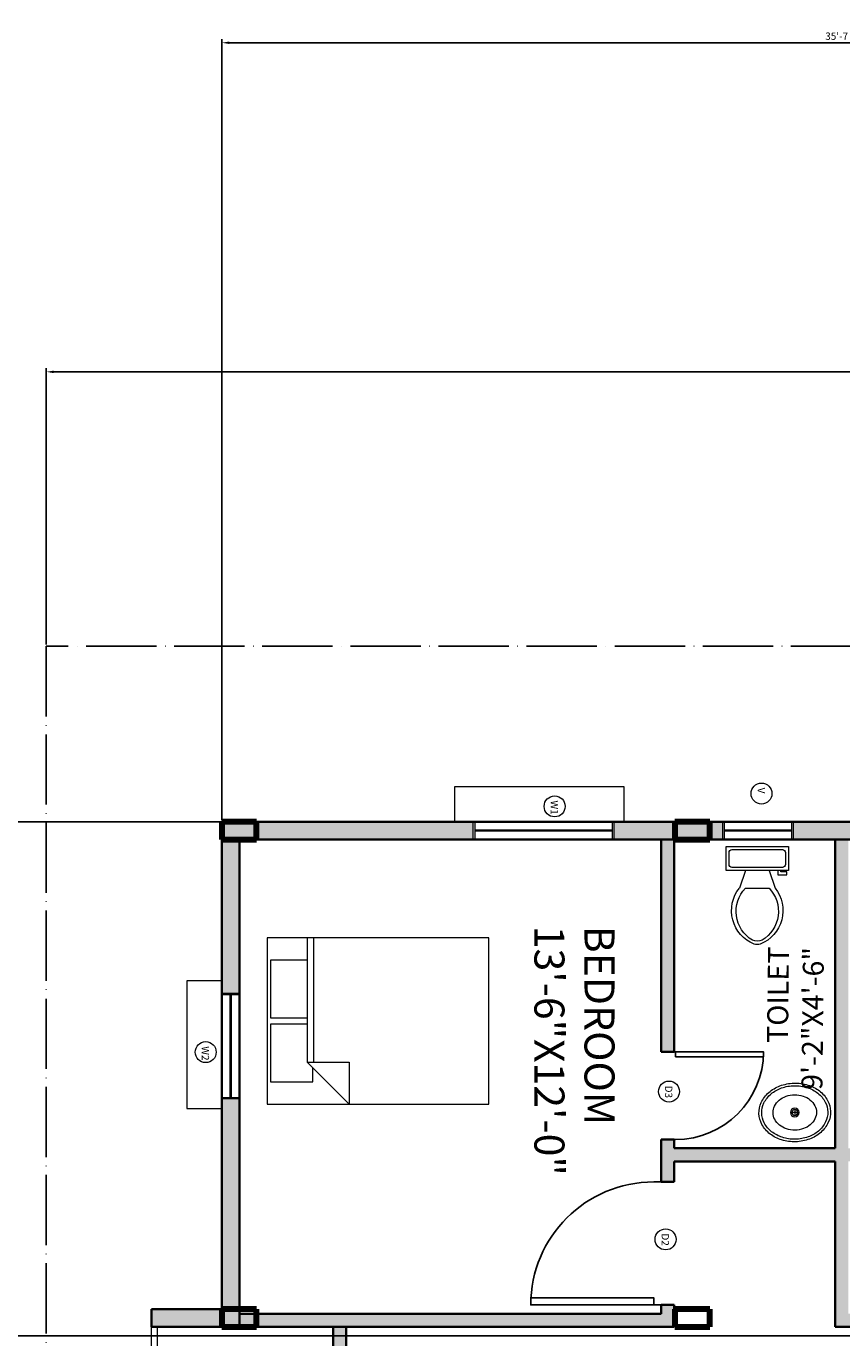
# Model space of a CAD drawing. Units: inches. Extents: x 7028582 to 7030319, y 63109697 to 63111305.
# Tile 11 of 18: x 7029168 to 7029446, y 63110857 to 63111305. Entities that reach past the tile are written whole.
import ezdxf

# ---------------------------------------------------------------- set-up
doc = ezdxf.new("R2010")
doc.units = ezdxf.units.IN
doc.linetypes.add('ACAD_ISO04W100', pattern=[30, 24, -3, 0, -3])
for name, color, linetype, lineweight in [('A-AREA-IDEN', 7, 'Continuous', 18), ('A-DOOR-IDEN', 20, 'Continuous', 13), ('A-FLOR-FIXT', 9, 'Continuous', 18), ('A-FLOR-HRAL', 5, 'Continuous', 18), ('A-GLAZ-IDEN', 20, 'Continuous', 13), ('A-WALL-PATT', 8, 'Continuous', 13), ('C-ANNO-DIMS', 7, 'Continuous', 18), ('C-PROP', 1, 'ACAD_ISO04W100', 25), ('doors', 20, 'Continuous', 25), ('furniture', 9, 'Continuous', 18), ('PILLARS', 220, 'Continuous', 100), ('S-COLS-PATT', 220, 'Continuous', 100), ('walls', 6, 'Continuous', 35), ('WINDOW SHADOW', 9, 'Continuous', 13), ('windows', 5, 'Continuous', 18)]:
    doc.layers.add(name, color=color, linetype=linetype, lineweight=lineweight)
doc.styles.get("Standard").update_dxf_attribs({"font": 'arial.ttf'})
doc.dimstyles.new('ISO-25', dxfattribs={"dimtxt": 2.5, "dimasz": 2.5, "dimexe": 1.25, "dimexo": 0.625, "dimtad": 1, "dimlunit": 4, "dimtxsty": 'Standard', "dimcen": 2.5, "dimadec": 0, "dimazin": 0, "dimtfac": 1, "dimtmove": 0, "dimatfit": 3, "dimfxl": 1, "dimarcsym": 0})

# ---------------------------------------------------------------- blocks, each defined once
blk = doc.blocks.new('*U2')
for p, q in [((0, 0), (0, -5)), ((30, 0), (30, -5))]:
    blk.add_line(p, q)
blk.add_lwpolyline([(0, 0), (0, 30), (1.75, 30), (1.75, 0)], close=True)
blk.add_arc((0, 0), 30, 0, 90)
blk = doc.blocks.new('Toilet - top')
for p, q in [((9.5, -6), (9.5, -2)), ((-10, -8.5), (-8, -8.5)), ((-10, -9.5), (-10, -8.5)), ((-8, -8.5), (-8, -8)), ((-7, -8), (-7, -9.5)), ((-4, -8), (-6, -14)), ((4, -8), (6, -14)), ((-7, -9.5), (-10, -9.5)), ((4, -14), (-4, -14))]:
    blk.add_line(p, q)
blk.add_lwpolyline([(10.5, -8), (10.5, 0), (-10.5, 0), (-10.5, -8)], close=True)
for points in [[(-9.5, -2), (-9.5, -6)], [(8.5, -1), (-8.5, -1)], [(-8.5, -7), (8.5, -7)]]:
    blk.add_lwpolyline(points)
for centre, radius, start, end in [((-8.62, -1.88), 0.884, 81.8699, 188.1301), ((8.62, -1.88), 0.884, 351.8699, 98.1301), ((-8.62, -6.12), 0.884, 171.8699, 278.1301), ((8.62, -6.12), 0.884, 261.8699, 8.1301), ((3.52, -21.58), 12.17, 141.4691, 247.9714), ((4.2, -21.82), 11.33, 136.3677, 238.9468), ((-3.52, -21.58), 12.17, 292.0284, 38.5307), ((-4.2, -21.82), 11.33, 301.053, 43.6321), ((0, -27.88), 4, 245.7318, 294.2682), ((0, -29), 4, 254.8605, 285.1395)]:
    blk.add_arc(centre, radius, start, end)
blk = doc.blocks.new('Sink - Oval top')
for p, q in [((-1, 0), (1, 0)), ((0, 1), (0, -1))]:
    blk.add_line(p, q)
for points in [[(-12.23, 0.39, 0.117634), (-11.46, -3.36, 0.104469), (-8.88, -6.8, 0.090016), (-5.08, -9.07, 0.08192), (-0.32, -10.02, 0.08192), (4.49, -9.38, 0.090016), (8.42, -7.36, 0.104469), (11.22, -4.09, 0.117634), (12.23, -0.39, 0.117634), (11.46, 3.36, 0.104469), (8.88, 6.8, 0.090016), (5.08, 9.07, 0.08192), (0.32, 10.02, 0.08192), (-4.49, 9.38, 0.090016), (-8.42, 7.36, 0.104469), (-11.22, 4.09, 0.117634)], [(-11.29, 0.16, 0.118622), (-10.52, -3.25, 0.104678), (-8.07, -6.36, 0.089562), (-4.54, -8.37, 0.081185), (-0.13, -9.15, 0.081185), (4.3, -8.49, 0.089562), (7.89, -6.58, 0.104678), (10.42, -3.55, 0.118622), (11.29, -0.16, 0.118622), (10.52, 3.25, 0.104678), (8.07, 6.36, 0.089562), (4.54, 8.37, 0.081185), (0.13, 9.15, 0.081185), (-4.3, 8.49, 0.089562), (-7.89, 6.58, 0.104678), (-10.42, 3.55, 0.118622)], [(-7.42, 0.08, 0.118283), (-6.91, -2.17, 0.104607), (-5.29, -4.21, 0.089718), (-2.97, -5.53, 0.081436), (-0.07, -6.04, 0.081436), (2.84, -5.59, 0.089718), (5.2, -4.33, 0.104607), (6.86, -2.32, 0.118283), (7.42, -0.08, 0.118283), (6.91, 2.17, 0.104607), (5.29, 4.21, 0.089718), (2.97, 5.53, 0.081436), (0.07, 6.04, 0.081436), (-2.84, 5.59, 0.089718), (-5.2, 4.33, 0.104607), (-6.86, 2.32, 0.118283)]]:
    blk.add_lwpolyline(points, format="xyb", close=True)
for radius in [1.5, 1]:
    blk.add_circle((0, 0), radius)
blk = doc.blocks.new('Bed - Queen')
for p, q in [((0, -80.00003), (0, 0)), ((0, 0), (59.99999, 0)), ((59.99999, 0), (59.99999, -80.00003)), ((7.99999, -1.2), (28.79998, -1.2)), ((7.99999, -14.4), (7.99999, -1.2)), ((28.79998, -1.2), (28.79998, -14.4)), ((31.19999, -1.2), (51.99999, -1.2)), ((31.19999, -14.4), (31.19999, -1.2)), ((51.99999, -1.2), (51.99999, -16.4)), ((0, -14.4), (44.8, -14.4)), ((44.8, -16.8), (0, -16.8)), ((59.99999, -29.6), (44.8, -14.4)), ((44.8, -14.4), (44.8, -29.6)), ((51.99999, -16.4), (46.79936, -16.4)), ((44.8, -29.6), (59.99999, -29.6)), ((59.99999, -80.00003), (0, -80.00003))]:
    blk.add_line(p, q)
blk = doc.blocks.new('*D11')
at = {"layer": 'C-ANNO-DIMS', "color": 0, "lineweight": -2, "transparency": 16777216}
for p, q in [((7029174.71, 63111093.68), (7029174.71, 63111188.03)), ((7030233.21, 63111186.78), (7029177.21, 63111186.78)), ((7030235.71, 63111093.68), (7030235.71, 63111188.03))]:
    blk.add_line(p, q, dxfattribs=at)
at = {"layer": 'C-ANNO-DIMS', "color": 0, "lineweight": 100, "transparency": 16777216}
for points in [[(7029177.21, 63111187.2), (7029177.21, 63111186.36), (7029174.71, 63111186.78)], [(7030233.21, 63111187.2), (7030233.21, 63111186.36), (7030235.71, 63111186.78)]]:
    blk.add_solid(points, dxfattribs=at)
at = {"layer": 'Defpoints', "color": 0, "lineweight": 100, "transparency": 16777216}
for p in [(7029174.71, 63111186.78), (7029174.71, 63111093.06), (7030235.71, 63111093.06)]:
    blk.add_point(p, dxfattribs=at)
at = {"layer": 'C-ANNO-DIMS', "color": 0, "transparency": 16777216, "insert": (7029705.21, 63111193.53), "char_height": 12, "attachment_point": 5}
blk.add_mtext('88\'-5"', dxfattribs=at)
blk = doc.blocks.new('WIN-SASH-36')
for p, q in [((0, 36.05), (0, 0)), ((6, 0), (6, 36.05)), ((6, 35.55), (0, 35.55)), ((2.8, 35.55), (2.8, 0.5)), ((3.2, 35.55), (3.2, 0.5)), ((0, 0.5), (6, 0.5))]:
    blk.add_line(p, q)
blk = doc.blocks.new('WIN-SASH-24')
for p, q in [((24.05, 6), (0, 6)), ((0.5, 6), (0.5, 0)), ((23.55, 0), (23.55, 6)), ((0, 0), (24.05, 0)), ((23.55, 3.2), (0.5, 3.2)), ((23.55, 2.8), (0.5, 2.8))]:
    blk.add_line(p, q)
blk = doc.blocks.new('WIN-SASH-48')
for p, q in [((48.05, 6), (0, 6)), ((0.5, 6), (0.5, 0)), ((47.55, 0), (47.55, 6)), ((47.55, 3.2), (0.5, 3.2)), ((47.55, 2.8), (0.5, 2.8)), ((0, 0), (48.05, 0))]:
    blk.add_line(p, q)
blk = doc.blocks.new('WINDOW-SHADE-SIDE-44')
for p, q in [((12, 43.55), (0, 43.55)), ((12, 0), (12, 43.55)), ((0, 0), (12, 0))]:
    blk.add_line(p, q)
blk = doc.blocks.new('WINDOW-SHADE-HEAD-58')
for p, q in [((57.96, 12), (0, 12)), ((0, 12), (0, 0)), ((57.96, 0), (57.96, 12))]:
    blk.add_line(p, q)
blk = doc.blocks.new('COLUMN-RECT-PROFILE')
for p, q in [((11.91, 6), (0, 6)), ((0, 6), (0, 0)), ((11.91, 0), (11.91, 6)), ((0, 0), (11.91, 0))]:
    blk.add_line(p, q)
blk = doc.blocks.new('BALCONY-GUARD-12FT')
for p, q in [((0, 144), (0, 0)), ((2, 144), (2, 0))]:
    blk.add_line(p, q)
blk = doc.blocks.new('TAG-D2-MT-L')
blk.add_circle((3.58, 3.58), 3.58)
at = {"insert": (2.23, 5.6), "char_height": 2.5, "attachment_point": 7, "rotation": 270}
blk.add_mtext_dynamic_manual_height_columns('D2', width=2.5021, gutter_width=12.5, heights=[0], dxfattribs=at)
blk = doc.blocks.new('TAG-D3-MT-L')
blk.add_circle((3.58, 3.58), 3.58)
at = {"insert": (2.23, 5.6), "char_height": 2.5, "attachment_point": 7, "rotation": 270}
blk.add_mtext_dynamic_manual_height_columns('D3', width=2.5021, gutter_width=12.5, heights=[0], dxfattribs=at)
blk = doc.blocks.new('TAG-V-MT-L')
blk.add_circle((3.58, 3.58), 3.58)
at = {"insert": (2.23, 5.6), "char_height": 2.5, "attachment_point": 7, "rotation": 270}
blk.add_mtext_dynamic_manual_height_columns('V', width=2.5021, gutter_width=12.5, heights=[0], dxfattribs=at)
blk = doc.blocks.new('TAG-W1-MT-L')
blk.add_circle((3.58, 3.58), 3.58)
at = {"insert": (2.23, 5.6), "char_height": 2.5, "attachment_point": 7, "rotation": 270}
blk.add_mtext_dynamic_manual_height_columns('W1', width=2.5021, gutter_width=12.5, heights=[0], dxfattribs=at)
blk = doc.blocks.new('TAG-W2-MT-L')
blk.add_circle((3.58, 3.58), 3.58)
at = {"insert": (2.23, 5.6), "char_height": 2.5, "attachment_point": 7, "rotation": 270}
blk.add_mtext_dynamic_manual_height_columns('W2', width=2.5021, gutter_width=12.5, heights=[0], dxfattribs=at)
blk = doc.blocks.new('*D100')
at = {"layer": 'C-ANNO-DIMS', "color": 0, "lineweight": -2, "transparency": 16777216}
for p, q in [((7029234.08, 63111033.06), (7028586.23, 63111033.06)), ((7028587.48, 63109969.06), (7028587.48, 63111030.56)), ((7029234.08, 63109966.56), (7028586.23, 63109966.56))]:
    blk.add_line(p, q, dxfattribs=at)
at = {"layer": 'C-ANNO-DIMS', "color": 0, "lineweight": 100, "transparency": 16777216}
for points in [[(7028587.06, 63111030.56), (7028587.89, 63111030.56), (7028587.48, 63111033.06)], [(7028587.06, 63109969.06), (7028587.89, 63109969.06), (7028587.48, 63109966.56)]]:
    blk.add_solid(points, dxfattribs=at)
at = {"layer": 'Defpoints', "color": 0, "lineweight": 100, "transparency": 16777216}
for p in [(7028587.48, 63111033.06), (7029234.71, 63111033.06), (7029234.71, 63109966.56)]:
    blk.add_point(p, dxfattribs=at)
at = {"layer": 'C-ANNO-DIMS', "color": 0, "transparency": 16777216, "insert": (7028585.56, 63110499.81), "char_height": 2.5, "attachment_point": 5, "rotation": 90}
blk.add_mtext('88\'-10 1/2"', dxfattribs=at)
blk = doc.blocks.new('*D104')
at = {"layer": 'C-ANNO-DIMS', "color": 0, "lineweight": -2, "transparency": 16777216}
for p, q in [((7029747.58, 63110857.56), (7028586.23, 63110857.56)), ((7028587.48, 63110812.06), (7028587.48, 63110855.06)), ((7029747.58, 63110809.56), (7028586.23, 63110809.56))]:
    blk.add_line(p, q, dxfattribs=at)
at = {"layer": 'C-ANNO-DIMS', "color": 0, "lineweight": 100, "transparency": 16777216}
for points in [[(7028587.06, 63110855.06), (7028587.89, 63110855.06), (7028587.48, 63110857.56)], [(7028587.06, 63110812.06), (7028587.89, 63110812.06), (7028587.48, 63110809.56)]]:
    blk.add_solid(points, dxfattribs=at)
at = {"layer": 'Defpoints', "color": 0, "lineweight": 100, "transparency": 16777216}
for p in [(7028587.48, 63110857.56), (7029748.21, 63110857.56), (7029748.21, 63110809.56)]:
    blk.add_point(p, dxfattribs=at)
at = {"layer": 'C-ANNO-DIMS', "color": 0, "transparency": 16777216, "insert": (7028585.57, 63110833.56), "char_height": 2.5, "attachment_point": 5, "rotation": 90}
blk.add_mtext('4\'-0"', dxfattribs=at)
blk = doc.blocks.new('*D111')
at = {"layer": 'C-ANNO-DIMS', "color": 0, "lineweight": -2, "transparency": 16777216}
for p, q in [((7029234.71, 63111033.68), (7029234.71, 63111300.44)), ((7029237.21, 63111299.19), (7029659.71, 63111299.19)), ((7029662.21, 63111033.68), (7029662.21, 63111300.44))]:
    blk.add_line(p, q, dxfattribs=at)
at = {"layer": 'C-ANNO-DIMS', "color": 0, "lineweight": 100, "transparency": 16777216}
for points in [[(7029237.21, 63111299.61), (7029237.21, 63111298.77), (7029234.71, 63111299.19)], [(7029659.71, 63111299.61), (7029659.71, 63111298.77), (7029662.21, 63111299.19)]]:
    blk.add_solid(points, dxfattribs=at)
at = {"layer": 'Defpoints', "color": 0, "lineweight": 100, "transparency": 16777216}
for p in [(7029662.21, 63111299.19), (7029234.71, 63111033.06), (7029662.21, 63111033.06)]:
    blk.add_point(p, dxfattribs=at)
at = {"layer": 'C-ANNO-DIMS', "color": 0, "transparency": 16777216, "insert": (7029448.46, 63111301.11), "char_height": 2.5, "attachment_point": 5}
blk.add_mtext('35\'-7 1/2"', dxfattribs=at)
blk = doc.blocks.new('*D112')
at = {"layer": 'C-ANNO-DIMS', "color": 0, "lineweight": -2, "transparency": 16777216}
for p, q in [((7029747.58, 63111033.06), (7028586.23, 63111033.06)), ((7028587.48, 63111030.56), (7028587.48, 63110548.06)), ((7029747.58, 63110545.56), (7028586.23, 63110545.56))]:
    blk.add_line(p, q, dxfattribs=at)
at = {"layer": 'C-ANNO-DIMS', "color": 0, "lineweight": 100, "transparency": 16777216}
for points in [[(7028587.06, 63111030.56), (7028587.89, 63111030.56), (7028587.48, 63111033.06)], [(7028587.06, 63110548.06), (7028587.89, 63110548.06), (7028587.48, 63110545.56)]]:
    blk.add_solid(points, dxfattribs=at)
at = {"layer": 'Defpoints', "color": 0, "lineweight": 100, "transparency": 16777216}
for p in [(7029748.21, 63111033.06), (7028587.48, 63110545.56), (7029748.21, 63110545.56)]:
    blk.add_point(p, dxfattribs=at)
at = {"layer": 'C-ANNO-DIMS', "color": 0, "transparency": 16777216, "insert": (7028585.56, 63110789.31), "char_height": 2.5, "attachment_point": 5, "rotation": 90}
blk.add_mtext('40\'-7 1/2"', dxfattribs=at)

msp = doc.modelspace()

# ---------------------------------------------------------------- hatches: boundary and pattern name
at = {"layer": 'A-WALL-PATT'}
h = msp.add_hatch(color=256, dxfattribs=at)
h.dxf.hatch_style = 1
h.paths.add_polyline_path([(7029234.705, 63111033.057), (7029320.549, 63111033.057), (7029320.549, 63111027.057), (7029240.705, 63111027.057), (7029240.705, 63110974.515), (7029234.705, 63110974.515)])
h = msp.add_hatch(color=256, dxfattribs=at)
h.dxf.hatch_style = 1
h.paths.add_polyline_path([(7029368.597, 63111033.057), (7029405.832, 63111033.057), (7029405.832, 63111027.057), (7029368.597, 63111027.057)])
h.paths.add_polyline_path([(7029384.705, 63111027.057), (7029389.205, 63111027.057), (7029389.205, 63110954.557), (7029384.705, 63110954.557)], flags=0)
h = msp.add_hatch(color=256, dxfattribs=at)
h.dxf.hatch_style = 1
h.paths.add_polyline_path([(7029429.881, 63111027.057), (7029466.152, 63111027.057), (7029466.152, 63111033.057), (7029429.881, 63111033.057)])
h = msp.add_hatch(color=256, dxfattribs=at)
h.dxf.hatch_style = 1
h.paths.add_polyline_path([(7029384.705, 63111027.057), (7029389.205, 63111027.057), (7029389.205, 63110954.557), (7029384.705, 63110954.557)], flags=0)
h.paths.add_polyline_path([(7029384.705, 63110924.557), (7029389.205, 63110924.557), (7029389.205, 63110921.557), (7029444.205, 63110921.557), (7029444.205, 63111027.057), (7029448.705, 63111027.057), (7029448.705, 63110921.557), (7029469.705, 63110921.557), (7029469.705, 63110917.057), (7029448.705, 63110917.057), (7029448.705, 63110865.057), (7029526.726, 63110865.057), (7029526.726, 63110860.557), (7029444.205, 63110860.557), (7029444.205, 63110917.057), (7029389.205, 63110917.057), (7029389.205, 63110910.057), (7029384.705, 63110910.057)])
h = msp.add_hatch(color=256, dxfattribs=at)
h.dxf.hatch_style = 1
h.paths.add_polyline_path([(7029389.205, 63111027.057), (7029384.705, 63111027.057), (7029384.705, 63110954.557), (7029389.205, 63110954.557)])
h = msp.add_hatch(color=256, dxfattribs=at)
h.dxf.hatch_style = 1
h.paths.add_polyline_path([(7029234.705, 63110938.466), (7029240.705, 63110938.466), (7029240.705, 63110860.557), (7029234.705, 63110860.557)])
h = msp.add_hatch(color=256, dxfattribs=at)
h.dxf.hatch_style = 1
h.paths.add_polyline_path([(7029210.705, 63110866.557), (7029234.705, 63110866.557), (7029234.705, 63110860.557), (7029210.705, 63110860.557)])
h = msp.add_hatch(color=256, dxfattribs=at)
h.dxf.hatch_style = 1
h.paths.add_polyline_path([(7029240.705, 63110865.057), (7029384.705, 63110865.057), (7029384.705, 63110868.057), (7029389.205, 63110868.057), (7029389.205, 63110860.557), (7029240.705, 63110860.557)])
h = msp.add_hatch(color=256, dxfattribs=at)
h.dxf.hatch_style = 1
h.paths.add_polyline_path([(7029272.705, 63110860.557), (7029277.205, 63110860.557), (7029277.205, 63110822.163), (7029272.705, 63110822.163)])
at = {"layer": 'S-COLS-PATT'}
h = msp.add_hatch(color=256, dxfattribs=at)
h.dxf.hatch_style = 1
h.paths.add_polyline_path([(7029246.574, 63111033.057), (7029234.705, 63111033.057), (7029234.705, 63111027.057), (7029246.574, 63111027.057)])
h = msp.add_hatch(color=256, dxfattribs=at)
h.dxf.hatch_style = 1
h.paths.add_polyline_path([(7029246.574, 63111033.057), (7029234.705, 63111033.057), (7029234.705, 63111027.057), (7029246.574, 63111027.057)])
h = msp.add_hatch(color=256, dxfattribs=at)
h.dxf.hatch_style = 1
h.paths.add_polyline_path([(7029401.355, 63111033.057), (7029389.44, 63111033.057), (7029389.44, 63111027.057), (7029401.355, 63111027.057)])
h = msp.add_hatch(color=256, dxfattribs=at)
h.dxf.hatch_style = 1
h.paths.add_polyline_path([(7029401.355, 63111033.057), (7029389.44, 63111033.057), (7029389.44, 63111027.057), (7029401.355, 63111027.057)])

# ---------------------------------------------------------------- linework, layer by layer
at = {"layer": 'C-PROP'}
for p, q in [((7029174.705, 63111093.057), (7029174.705, 63109906.557)), ((7030235.705, 63111093.057), (7029174.705, 63111093.057))]:
    msp.add_line(p, q, dxfattribs=at)
at = {"layer": 'PILLARS'}
for p, q in [((7029246.574, 63111033.057), (7029234.659, 63111033.057)), ((7029234.659, 63111033.057), (7029234.659, 63111027.057)), ((7029246.574, 63111027.057), (7029246.574, 63111033.057)), ((7029401.355, 63111033.057), (7029389.44, 63111033.057)), ((7029389.44, 63111033.057), (7029389.44, 63111027.057)), ((7029401.355, 63111027.057), (7029401.355, 63111033.057)), ((7029234.659, 63111027.057), (7029246.574, 63111027.057)), ((7029389.44, 63111027.057), (7029401.355, 63111027.057))]:
    msp.add_line(p, q, dxfattribs=at)
at = {"layer": 'walls'}
for p, q in [((7030175.705, 63111033.057), (7029234.705, 63111033.057)), ((7029234.705, 63111033.057), (7029234.705, 63110860.557)), ((7029234.705, 63110860.557), (7029234.705, 63111033.057)), ((7029234.705, 63111033.057), (7030175.705, 63111033.057)), ((7030169.705, 63111027.057), (7029240.705, 63111027.057)), ((7029240.705, 63111027.057), (7029240.705, 63110860.557)), ((7029240.705, 63110860.557), (7029240.705, 63111027.057)), ((7029240.705, 63111027.057), (7030169.705, 63111027.057)), ((7029384.705, 63110954.557), (7029384.705, 63111027.057)), ((7029389.205, 63110954.557), (7029389.205, 63111027.057)), ((7029444.205, 63110921.557), (7029444.205, 63111027.057)), ((7029384.705, 63110954.557), (7029389.205, 63110954.557)), ((7029384.705, 63110910.057), (7029384.705, 63110924.557)), ((7029389.205, 63110924.557), (7029384.705, 63110924.557)), ((7029389.205, 63110921.557), (7029389.205, 63110924.557)), ((7029389.205, 63110921.557), (7029389.205, 63110924.557)), ((7029389.205, 63110921.557), (7029444.205, 63110921.557)), ((7029389.205, 63110910.057), (7029389.205, 63110917.057)), ((7029389.205, 63110917.057), (7029444.205, 63110917.057)), ((7029444.205, 63110860.557), (7029444.205, 63110917.057)), ((7029389.205, 63110910.057), (7029384.705, 63110910.057)), ((7029210.705, 63110860.557), (7029210.705, 63110866.557)), ((7029210.705, 63110866.557), (7029234.705, 63110866.557)), ((7029240.705, 63110865.057), (7029384.705, 63110865.057)), ((7029384.705, 63110865.057), (7029384.705, 63110868.057)), ((7029384.705, 63110865.057), (7029384.705, 63110868.057)), ((7029384.705, 63110868.057), (7029389.205, 63110868.057)), ((7029389.205, 63110860.557), (7029389.205, 63110868.057)), ((7029234.705, 63110860.557), (7029210.705, 63110860.557)), ((7029234.705, 63110860.557), (7029389.205, 63110860.557)), ((7029272.705, 63110860.557), (7029272.705, 63110716.557)), ((7029277.205, 63110860.557), (7029277.205, 63110716.557)), ((7029444.205, 63110860.557), (7029526.726, 63110860.557))]:
    msp.add_line(p, q, dxfattribs=at)
at = {"layer": 'windows'}
for p, q in [((7029320.549, 63111027.057), (7029320.549, 63111033.057)), ((7029368.597, 63111033.057), (7029368.597, 63111027.057)), ((7029405.832, 63111027.057), (7029405.832, 63111033.057)), ((7029429.881, 63111033.057), (7029429.881, 63111027.057)), ((7029234.635, 63110974.515), (7029240.635, 63110974.515)), ((7029240.635, 63110938.466), (7029234.635, 63110938.466))]:
    msp.add_line(p, q, dxfattribs=at)

# ---------------------------------------------------------------- block references
at = {"layer": 'A-DOOR-IDEN'}
for name, p in [('TAG-D3-MT-L', (7029383.855, 63110937.359)), ('TAG-D2-MT-L', (7029382.689, 63110886.879))]:
    msp.add_blockref(name, p, dxfattribs=at)
at = {"layer": 'A-FLOR-FIXT', "xscale": -1.013555723357934, "yscale": 1.013555723357934, "zscale": 1.013555723357934}
msp.add_blockref('Toilet - top', (7029417.569, 63111024.605), dxfattribs=at)
at = {"layer": 'A-FLOR-FIXT', "xscale": -1}
msp.add_blockref('Sink - Oval top', (7029430.396, 63110933.801), dxfattribs=at)
at = {"layer": 'A-FLOR-HRAL', "rotation": 180}
msp.add_blockref('BALCONY-GUARD-12FT', (7029212.705, 63110860.557), dxfattribs=at)
at = {"layer": 'A-GLAZ-IDEN'}
for name, p in [('TAG-V-MT-L', (7029415.449, 63111039.151)), ('TAG-W1-MT-L', (7029344.79, 63111034.779)), ('TAG-W2-MT-L', (7029225.585, 63110950.827))]:
    msp.add_blockref(name, p, dxfattribs=at)
at = {"layer": 'doors', "rotation": 270}
msp.add_blockref('*U2', (7029389.705, 63110954.557), dxfattribs=at)
at = {"layer": 'doors', "xscale": 1.399999999999999, "yscale": 1.399999999999999, "zscale": 1.399999999999999, "rotation": 90.00000000000003}
msp.add_blockref('*U2', (7029382.205, 63110868.057), dxfattribs=at)
at = {"layer": 'furniture', "xscale": -0.9464141645025947, "yscale": 0.9464141645025947, "zscale": 0.9464141645025947, "rotation": 90}
msp.add_blockref('Bed - Queen', (7029250.204, 63110993.435), dxfattribs=at)
at = {"layer": 'PILLARS'}
for p in [(7029234.659, 63110860.557), (7029389.44, 63110860.557)]:
    msp.add_blockref('COLUMN-RECT-PROFILE', p, dxfattribs=at)
at = {"layer": 'WINDOW SHADOW'}
msp.add_blockref('WINDOW-SHADE-HEAD-58', (7029314.122, 63111033.057), dxfattribs=at)
at = {"layer": 'WINDOW SHADOW', "rotation": 180}
msp.add_blockref('WINDOW-SHADE-SIDE-44', (7029234.706, 63110978.719), dxfattribs=at)
at = {"layer": 'windows'}
for name, p in [('WIN-SASH-48', (7029320.549, 63111027.057)), ('WIN-SASH-24', (7029405.832, 63111027.057)), ('WIN-SASH-36', (7029234.635, 63110938.466))]:
    msp.add_blockref(name, p, dxfattribs=at)

# ---------------------------------------------------------------- texts
at = {"layer": 'A-AREA-IDEN'}
for s, width, gutter_width, insert, char_height, attachment_point, rotation in [('BEDROOM\\P13\'-6"X12\'-0"', 82.04322, 51.315, (7029341.455, 63110997.575), 10.26307, 7, 270), ('TOILET\\P9\'-2"X4\'-6"', 42.97461, 35.821, (7029421.278, 63110990.477), 7.16426, 3, 89.3536)]:
    msp.add_mtext_dynamic_manual_height_columns(s, width=width, gutter_width=gutter_width, heights=[0], dxfattribs=dict(at, insert=insert, char_height=char_height, attachment_point=attachment_point, rotation=rotation))

# ---------------------------------------------------------------- dimensions: what is measured, and where the dimension line sits
at = {"layer": 'C-ANNO-DIMS'}
for base, p1, p2, override, picture, middle in [((7029662.205, 63111299.19), (7029234.705, 63111033.057), (7029662.205, 63111033.057), {"dimdec": 1, "dimlfac": 1, "dimrnd": 0, "dimzin": 1, "dimdsep": 46, "dimlunit": 4, "dimfrac": 2}, '*D111', (7029448.455, 63111301.108)), ((7029174.705, 63111186.781), (7030235.705, 63111093.057), (7029174.705, 63111093.057), {"dimtxt": 12, "dimclrd": 0, "dimclre": 0, "dimclrt": 0}, '*D11', (7029705.205, 63111193.533))]:
    dim = msp.add_linear_dim(base=base, p1=p1, p2=p2, dimstyle='ISO-25', override=override, dxfattribs=at)
    dim.commit()
    dim.dimension.update_dxf_attribs({"geometry": picture, "text_midpoint": middle})
for base, p1, p2, picture, middle in [((7028587.475, 63111033.057), (7029234.705, 63109966.557), (7029234.705, 63111033.057), '*D100', (7028585.558, 63110499.807)), ((7028587.475, 63110545.557), (7029748.205, 63111033.057), (7029748.205, 63110545.557), '*D112', (7028585.558, 63110789.307)), ((7028587.475, 63110857.557), (7029748.205, 63110809.557), (7029748.205, 63110857.557), '*D104', (7028585.574, 63110833.557))]:
    dim = msp.add_linear_dim(base=base, p1=p1, p2=p2, angle=90, dimstyle='ISO-25', override={"dimdec": 1, "dimlfac": 1, "dimrnd": 0, "dimzin": 1, "dimdsep": 46, "dimlunit": 4, "dimfrac": 2}, dxfattribs=at)
    dim.commit()
    dim.dimension.update_dxf_attribs({"geometry": picture, "text_midpoint": middle})

doc.saveas('drawing.dxf')
